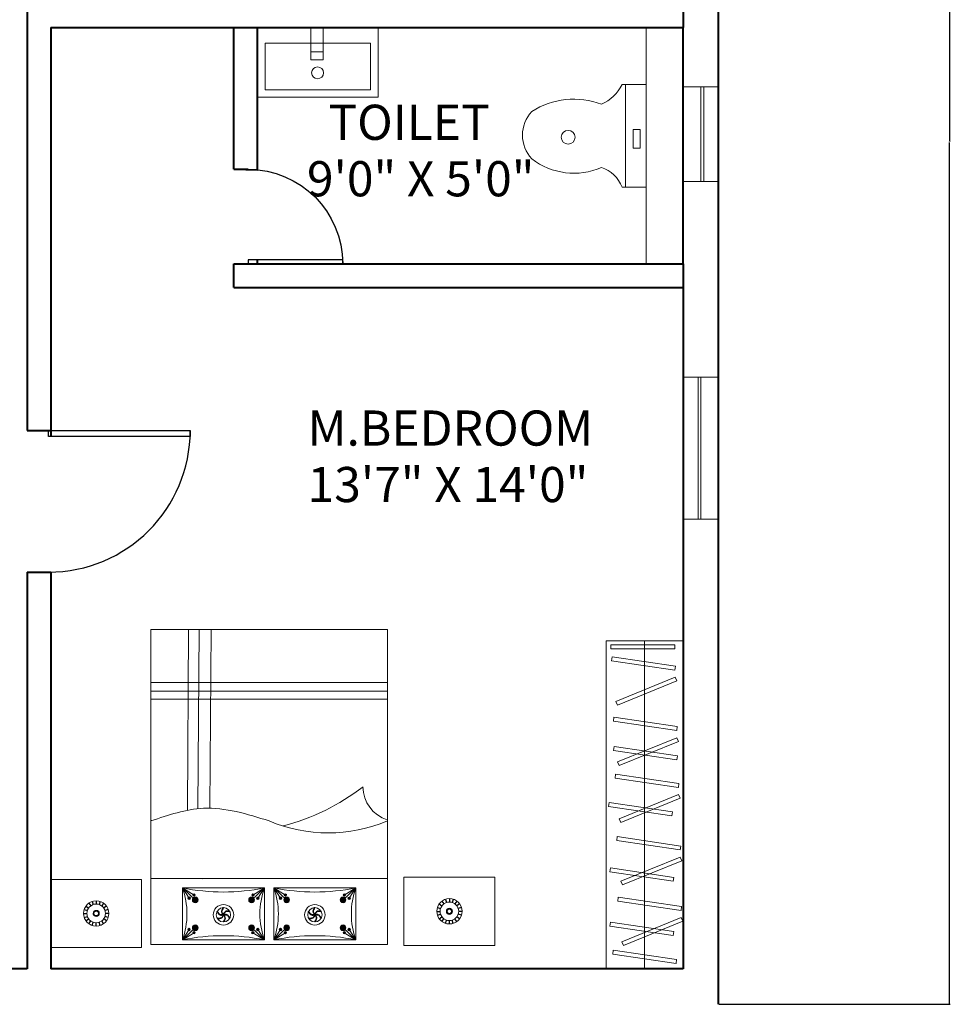
# Model space of a CAD drawing. Units: inches. Extents: x -46 to 1145, y -527 to 760.
# Tile 56 of 57: x 909 to 1145, y 222 to 472. Entities that reach past the tile are written whole.
import ezdxf

# ---------------------------------------------------------------- set-up
doc = ezdxf.new("R2010")
doc.units = ezdxf.units.IN
doc.header["$MEASUREMENT"] = 0
for name, color, linetype, lineweight in [('A-ANNO-DIMS', 2, 'Continuous', 18), ('A-AREA-IDEN', 1, 'Continuous', 18), ('A-FLOR-CASE', 32, 'Continuous', 18), ('A-FLOR-FIXT', 9, 'Continuous', 18), ('A-FURN', 2, 'Continuous', 13), ('DOORS', 3, 'Continuous', 25), ('WALLS', 4, 'Continuous', 40), ('WINDOWS', 240, 'Continuous', 20)]:
    doc.layers.add(name, color=color, linetype=linetype, lineweight=lineweight)
doc.layers.add('FURNTIURE', color=2, linetype='Continuous')
doc.layers.add('LT', color=9, linetype='Continuous')
doc.styles.get("Standard").update_dxf_attribs({"font": 'arial.ttf'})
doc.dimstyles.get("Standard").update_dxf_attribs({"dimtxt": 0.18, "dimasz": 0.18, "dimexe": 0.18, "dimexo": 0.0625, "dimgap": 0.09, "dimtad": 0, "dimtih": 1, "dimtoh": 1, "dimdec": 0, "dimzin": 0, "dimdsep": 46, "dimlunit": 3, "dimtxsty": 'Standard', "dimcen": 0.09, "dimadec": 0, "dimazin": 0, "dimtfac": 1, "dimtdec": 0, "dimtofl": 0, "dimtmove": 0, "dimatfit": 3, "dimfxl": 1, "dimtolj": 1, "dimtzin": 0, "dimarcsym": 0})

# ---------------------------------------------------------------- blocks, each defined once
blk = doc.blocks.new('*U2')
for p, q in [((0, 0), (0, -6)), ((40, 0), (40, -6))]:
    blk.add_line(p, q)
blk.add_lwpolyline([(0, 0), (0, 40), (1.75, 40), (1.75, 0)], close=True)
blk.add_arc((0, 0), 40, 0, 90)
blk = doc.blocks.new('*U89')
at = {"layer": 'FURNTIURE'}
blk.add_line((0, 0.42), (0, -0.42), dxfattribs=at)
blk = doc.blocks.new('*U90')
at = {"layer": 'FURNTIURE', "transparency": 16777216}
for p, rotation in [((590.89, 507.4), 17.99999999999997), ((592.61, 507.4), 341.9999999999999), ((589.1, 505.61), 72), ((589.5, 506.39), 54), ((590.11, 507), 36), ((593.39, 507), 324), ((594.01, 506.39), 306), ((594.4, 505.61), 288), ((588.97, 504.75), 90), ((589.1, 503.89), 108), ((589.5, 503.11), 126), ((590.11, 502.49), 144), ((590.89, 502.1), 162), ((592.61, 502.1), 197.9999999999999), ((593.39, 502.49), 216), ((594.01, 503.11), 234), ((594.4, 503.89), 252), ((594.54, 504.75), 270), ((591.75, 501.96), 180)]:
    blk.add_blockref('*U89', p, dxfattribs=dict(at, rotation=rotation))
blk.add_blockref('*U89', (591.75, 507.53), dxfattribs=at)
blk = doc.blocks.new('*U87')
at = {"layer": 'FURNTIURE'}
blk.add_line((0, 0.1), (0, -0.1), dxfattribs=at)
blk = doc.blocks.new('*U88')
at = {"layer": 'FURNTIURE', "transparency": 16777216}
for p, rotation in [((141.23, 121.04), 90), ((141.27, 121.25), 72), ((141.27, 120.83), 108), ((141.36, 121.43), 54), ((141.36, 120.65), 126), ((141.51, 121.58), 35.99999999999999), ((141.51, 120.5), 144), ((141.7, 121.67), 17.99999999999998), ((141.7, 120.4), 162), ((141.9, 120.37), 180), ((142.11, 121.67), 342), ((142.11, 120.4), 198), ((142.3, 121.58), 324), ((142.3, 120.5), 216), ((142.44, 121.43), 306), ((142.44, 120.65), 234), ((142.54, 121.25), 288), ((142.54, 120.83), 252), ((142.57, 121.04), 270)]:
    blk.add_blockref('*U87', p, dxfattribs=dict(at, rotation=rotation))
blk.add_blockref('*U87', (141.9, 121.71), dxfattribs=at)
blk = doc.blocks.new('NIGHTSTAND')
blk.add_lwpolyline([(23.06, 0), (0, 0), (0, 17.28), (23.06, 17.28)], close=True)
for radius in [3.21, 2.36, 0.77, 0.567]:
    blk.add_circle((11.53, 8.64), radius)
for name, p in [('*U90', (-580.22, -496.1)), ('*U88', (-130.37, -112.4))]:
    blk.add_blockref(name, p)
blk = doc.blocks.new('WARDROBE')
blk.add_line((9.78, 0), (9.78, 83.25))
for points in [[(19.56, 0), (0, 0), (0, 83.25), (19.56, 83.25)], [(17.74, 78.49), (1.66, 80.88), (1.8, 81.87), (17.88, 79.48)], [(15.55, 76.35), (0.49, 70.23), (0.11, 71.16), (15.17, 77.28)], [(18.43, 71.4), (2.35, 73.79), (2.5, 74.78), (18.58, 72.39)], [(16.47, 65.03), (0.39, 67.42), (0.54, 68.41), (16.62, 66.02)], [(15.79, 61), (0.73, 54.88), (0.35, 55.81), (15.41, 61.93)], [(18.43, 57.62), (2.35, 60.01), (2.5, 61), (18.58, 58.61)], [(16.71, 49.68), (0.63, 52.07), (0.78, 53.06), (16.86, 50.67)], [(16.22, 45.12), (1.16, 39), (0.78, 39.93), (15.84, 46.05)], [(18.77, 41.02), (2.69, 43.41), (2.84, 44.4), (18.92, 42.01)], [(17.14, 33.8), (1.06, 36.19), (1.21, 37.19), (17.29, 34.8)], [(16.65, 30.67), (1.59, 24.55), (1.21, 25.48), (16.27, 31.6)], [(17.52, 26.78), (1.44, 29.17), (1.59, 30.16), (17.67, 27.77)], [(17.57, 19.35), (1.49, 21.74), (1.64, 22.73), (17.72, 20.34)], [(17.08, 15.35), (2.02, 9.23), (1.64, 10.16), (16.7, 16.28)], [(18, 4.03), (1.92, 6.42), (2.07, 7.41), (18.15, 5.03)], [(18.32, 0.98), (2.07, 0.98), (2.07, 1.98), (18.32, 1.98)]]:
    blk.add_lwpolyline(points, close=True)
blk = doc.blocks.new('LAVATORY-RECT')
blk.add_line((14.01, 6.17), (17.08, 6.17))
for points in [[(30.61, 0), (0, 0), (0, 17.7), (30.61, 17.7)], [(28.7, 3.94), (1.97, 3.94), (1.97, 15.81), (28.7, 15.81)], [(17.08, 0), (14.01, 0), (14.01, 8.17), (17.08, 8.17)]]:
    blk.add_lwpolyline(points, close=True)
blk.add_circle((15.39, 11.51), 1.51)
blk = doc.blocks.new('WATER-CLOSET')
for p, q in [((0, 0), (0, 26.01)), ((0, 26.01), (6.13, 26.01)), ((5.22, 21.04), (5.22, 26.01)), ((5.22, 26.01), (5.22, 0)), ((0, 0), (6.13, 0))]:
    blk.add_line(p, q)
blk.add_lwpolyline([(1.51, 11.4), (1.51, 16.16), (3.34, 16.16), (3.34, 11.4)], close=True)
blk.add_circle((19.79, 13.37), 1.75)
for centre, radius, start, end in [((14.15, 29.2), 8.64, 201.6782, 251.0259), ((18.35, 4.96), 17.54, 52.4616, 113.5359), ((22.52, 12.84), 8.87, 317.2682, 42.7318), ((18.33, 23.71), 20, 249.5645, 302.3709), ((15.4, -4.5), 10.31, 113.1704, 154.0947)]:
    blk.add_arc(centre, radius, start, end)
blk = doc.blocks.new('WINDOW-36IN')
for p, q in [((0, 4.5), (0, 9)), ((0, 9), (0, 0)), ((36, 9), (36, 0)), ((0, 5.23), (36, 5.23)), ((0, 4.5), (36, 4.5))]:
    blk.add_line(p, q)
blk = doc.blocks.new('WINDOW-24IN')
for p, q in [((0, 4.5), (0, 9)), ((0, 9), (0, 0)), ((24, 9), (24, 0)), ((0, 5.23), (24, 5.23)), ((0, 4.5), (24, 4.5))]:
    blk.add_line(p, q)
blk = doc.blocks.new('*U58')
at = {"layer": 'LT'}
blk.add_line((0, 0.28), (0, -0.28), dxfattribs=at)
for centre, start, end in [((0.73, 0), 159.0676, 200.9324), ((-0.73, 0), 339.0676, 20.9324)]:
    blk.add_arc(centre, 0.786, start, end, dxfattribs=at)
blk = doc.blocks.new('*U59')
at = {"layer": 'LT', "transparency": 16777216}
for p, rotation in [((609.66, 443.79), 80.00000000000001), ((609.69, 443.6), 120), ((609.76, 443.96), 40.00000000000002), ((609.84, 443.48), 160), ((610.03, 443.48), 200), ((610.12, 443.96), 320), ((610.18, 443.6), 240), ((610.21, 443.79), 280)]:
    blk.add_blockref('*U58', p, dxfattribs=dict(at, rotation=rotation))
blk.add_blockref('*U58', (609.94, 444.03), dxfattribs=at)
blk = doc.blocks.new('*U60')
at = {"layer": 'LT'}
blk.add_line((0, 0.12), (0, -0.12), dxfattribs=at)
for centre, start, end in [((0.31, 0), 159.0676, 200.9324), ((-0.31, 0), 339.0676, 20.9324)]:
    blk.add_arc(centre, 0.335, start, end, dxfattribs=at)
blk = doc.blocks.new('*U61')
at = {"layer": 'LT', "transparency": 16777216}
for p, rotation in [((259.5, 188.9), 80.00000000000001), ((259.51, 188.82), 120), ((259.54, 188.97), 40), ((259.57, 188.76), 160), ((259.65, 188.76), 200), ((259.69, 188.97), 320), ((259.72, 188.82), 240), ((259.73, 188.9), 280)]:
    blk.add_blockref('*U60', p, dxfattribs=dict(at, rotation=rotation))
blk.add_blockref('*U60', (259.61, 189), dxfattribs=at)
blk = doc.blocks.new('*U62')
at = {"layer": 'LT'}
blk.add_line((0, 0.12), (0, -0.12), dxfattribs=at)
for centre, start, end in [((0.31, 0), 159.0676, 200.9324), ((-0.31, 0), 339.0676, 20.9324)]:
    blk.add_arc(centre, 0.335, start, end, dxfattribs=at)
blk = doc.blocks.new('*U63')
at = {"layer": 'LT', "transparency": 16777216}
for p, rotation in [((259.5, 188.9), 80.00000000000001), ((259.51, 188.82), 120), ((259.54, 188.97), 40), ((259.57, 188.76), 160), ((259.65, 188.76), 200), ((259.69, 188.97), 320), ((259.72, 188.82), 240), ((259.73, 188.9), 280)]:
    blk.add_blockref('*U62', p, dxfattribs=dict(at, rotation=rotation))
blk.add_blockref('*U62', (259.61, 189), dxfattribs=at)
blk = doc.blocks.new('*U64')
at = {"layer": 'LT'}
blk.add_line((0, 0.28), (0, -0.28), dxfattribs=at)
for centre, start, end in [((0.73, 0), 159.0676, 200.9324), ((-0.73, 0), 339.0676, 20.9324)]:
    blk.add_arc(centre, 0.786, start, end, dxfattribs=at)
blk = doc.blocks.new('*U65')
at = {"layer": 'LT', "transparency": 16777216}
for p, rotation in [((609.66, 443.79), 80.00000000000001), ((609.69, 443.6), 120), ((609.76, 443.96), 40.00000000000002), ((609.84, 443.48), 160), ((610.03, 443.48), 200), ((610.12, 443.96), 320), ((610.18, 443.6), 240), ((610.21, 443.79), 280)]:
    blk.add_blockref('*U64', p, dxfattribs=dict(at, rotation=rotation))
blk.add_blockref('*U64', (609.94, 444.03), dxfattribs=at)
blk = doc.blocks.new('*U66')
at = {"layer": 'LT'}
blk.add_line((0, 0.12), (0, -0.12), dxfattribs=at)
for centre, start, end in [((0.31, 0), 159.0676, 200.9324), ((-0.31, 0), 339.0676, 20.9324)]:
    blk.add_arc(centre, 0.335, start, end, dxfattribs=at)
blk = doc.blocks.new('*U67')
at = {"layer": 'LT', "transparency": 16777216}
for p, rotation in [((259.5, 188.9), 80.00000000000001), ((259.51, 188.82), 120), ((259.54, 188.97), 40), ((259.57, 188.76), 160), ((259.65, 188.76), 200), ((259.69, 188.97), 320), ((259.72, 188.82), 240), ((259.73, 188.9), 280)]:
    blk.add_blockref('*U66', p, dxfattribs=dict(at, rotation=rotation))
blk.add_blockref('*U66', (259.61, 189), dxfattribs=at)
blk = doc.blocks.new('*U68')
at = {"layer": 'LT'}
blk.add_line((0, 0.12), (0, -0.12), dxfattribs=at)
for centre, start, end in [((0.31, 0), 159.0676, 200.9324), ((-0.31, 0), 339.0676, 20.9324)]:
    blk.add_arc(centre, 0.335, start, end, dxfattribs=at)
blk = doc.blocks.new('*U69')
at = {"layer": 'LT', "transparency": 16777216}
for p, rotation in [((259.5, 188.9), 80.00000000000001), ((259.51, 188.82), 120), ((259.54, 188.97), 40), ((259.57, 188.76), 160), ((259.65, 188.76), 200), ((259.69, 188.97), 320), ((259.72, 188.82), 240), ((259.73, 188.9), 280)]:
    blk.add_blockref('*U68', p, dxfattribs=dict(at, rotation=rotation))
blk.add_blockref('*U68', (259.61, 189), dxfattribs=at)
blk = doc.blocks.new('*U70')
at = {"layer": 'LT'}
blk.add_line((0, 0.28), (0, -0.28), dxfattribs=at)
for centre, start, end in [((0.73, 0), 159.0676, 200.9324), ((-0.73, 0), 339.0676, 20.9324)]:
    blk.add_arc(centre, 0.786, start, end, dxfattribs=at)
blk = doc.blocks.new('*U71')
at = {"layer": 'LT', "transparency": 16777216}
for p, rotation in [((609.66, 443.79), 80.00000000000001), ((609.69, 443.6), 120), ((609.76, 443.96), 40.00000000000002), ((609.84, 443.48), 160), ((610.03, 443.48), 200), ((610.12, 443.96), 320), ((610.18, 443.6), 240), ((610.21, 443.79), 280)]:
    blk.add_blockref('*U70', p, dxfattribs=dict(at, rotation=rotation))
blk.add_blockref('*U70', (609.94, 444.03), dxfattribs=at)
blk = doc.blocks.new('*U46')
at = {"layer": 'LT'}
blk.add_line((0, 0.12), (0, -0.12), dxfattribs=at)
for centre, start, end in [((0.31, 0), 159.0676, 200.9324), ((-0.31, 0), 339.0676, 20.9324)]:
    blk.add_arc(centre, 0.335, start, end, dxfattribs=at)
blk = doc.blocks.new('*U47')
at = {"layer": 'LT', "transparency": 16777216}
for p, rotation in [((259.5, 188.9), 80.00000000000001), ((259.51, 188.82), 120), ((259.54, 188.97), 40), ((259.57, 188.76), 160), ((259.65, 188.76), 200), ((259.69, 188.97), 320), ((259.72, 188.82), 240), ((259.73, 188.9), 280)]:
    blk.add_blockref('*U46', p, dxfattribs=dict(at, rotation=rotation))
blk.add_blockref('*U46', (259.61, 189), dxfattribs=at)
blk = doc.blocks.new('*U48')
at = {"layer": 'LT'}
blk.add_line((0, 0.12), (0, -0.12), dxfattribs=at)
for centre, start, end in [((0.31, 0), 159.0676, 200.9324), ((-0.31, 0), 339.0676, 20.9324)]:
    blk.add_arc(centre, 0.335, start, end, dxfattribs=at)
blk = doc.blocks.new('*U49')
at = {"layer": 'LT', "transparency": 16777216}
for p, rotation in [((259.5, 188.9), 80.00000000000001), ((259.51, 188.82), 120), ((259.54, 188.97), 40), ((259.57, 188.76), 160), ((259.65, 188.76), 200), ((259.69, 188.97), 320), ((259.72, 188.82), 240), ((259.73, 188.9), 280)]:
    blk.add_blockref('*U48', p, dxfattribs=dict(at, rotation=rotation))
blk.add_blockref('*U48', (259.61, 189), dxfattribs=at)
blk = doc.blocks.new('*U50')
at = {"layer": 'LT'}
blk.add_line((0, 0.28), (0, -0.28), dxfattribs=at)
for centre, start, end in [((0.73, 0), 159.0676, 200.9324), ((-0.73, 0), 339.0676, 20.9324)]:
    blk.add_arc(centre, 0.786, start, end, dxfattribs=at)
blk = doc.blocks.new('*U51')
at = {"layer": 'LT', "transparency": 16777216}
for p, rotation in [((609.66, 443.79), 80.00000000000001), ((609.69, 443.6), 120), ((609.76, 443.96), 40.00000000000002), ((609.84, 443.48), 160), ((610.03, 443.48), 200), ((610.12, 443.96), 320), ((610.18, 443.6), 240), ((610.21, 443.79), 280)]:
    blk.add_blockref('*U50', p, dxfattribs=dict(at, rotation=rotation))
blk.add_blockref('*U50', (609.94, 444.03), dxfattribs=at)
blk = doc.blocks.new('*U52')
at = {"layer": 'LT'}
blk.add_line((0, 0.12), (0, -0.12), dxfattribs=at)
for centre, start, end in [((0.31, 0), 159.0676, 200.9324), ((-0.31, 0), 339.0676, 20.9324)]:
    blk.add_arc(centre, 0.335, start, end, dxfattribs=at)
blk = doc.blocks.new('*U53')
at = {"layer": 'LT', "transparency": 16777216}
for p, rotation in [((259.5, 188.9), 80.00000000000001), ((259.51, 188.82), 120), ((259.54, 188.97), 40), ((259.57, 188.76), 160), ((259.65, 188.76), 200), ((259.69, 188.97), 320), ((259.72, 188.82), 240), ((259.73, 188.9), 280)]:
    blk.add_blockref('*U52', p, dxfattribs=dict(at, rotation=rotation))
blk.add_blockref('*U52', (259.61, 189), dxfattribs=at)
blk = doc.blocks.new('*U54')
at = {"layer": 'LT'}
blk.add_line((0, 0.12), (0, -0.12), dxfattribs=at)
for centre, start, end in [((0.31, 0), 159.0676, 200.9324), ((-0.31, 0), 339.0676, 20.9324)]:
    blk.add_arc(centre, 0.335, start, end, dxfattribs=at)
blk = doc.blocks.new('*U55')
at = {"layer": 'LT', "transparency": 16777216}
for p, rotation in [((259.5, 188.9), 80.00000000000001), ((259.51, 188.82), 120), ((259.54, 188.97), 40), ((259.57, 188.76), 160), ((259.65, 188.76), 200), ((259.69, 188.97), 320), ((259.72, 188.82), 240), ((259.73, 188.9), 280)]:
    blk.add_blockref('*U54', p, dxfattribs=dict(at, rotation=rotation))
blk.add_blockref('*U54', (259.61, 189), dxfattribs=at)
blk = doc.blocks.new('*U34')
at = {"layer": 'LT'}
blk.add_line((0, 0.28), (0, -0.28), dxfattribs=at)
for centre, start, end in [((0.73, 0), 159.0676, 200.9324), ((-0.73, 0), 339.0676, 20.9324)]:
    blk.add_arc(centre, 0.786, start, end, dxfattribs=at)
blk = doc.blocks.new('*U35')
at = {"layer": 'LT', "transparency": 16777216}
for p, rotation in [((609.66, 443.79), 80.00000000000001), ((609.69, 443.6), 120), ((609.76, 443.96), 40.00000000000002), ((609.84, 443.48), 160), ((610.03, 443.48), 200), ((610.12, 443.96), 320), ((610.18, 443.6), 240), ((610.21, 443.79), 280)]:
    blk.add_blockref('*U34', p, dxfattribs=dict(at, rotation=rotation))
blk.add_blockref('*U34', (609.94, 444.03), dxfattribs=at)
blk = doc.blocks.new('*U36')
at = {"layer": 'LT'}
blk.add_line((0, 0.12), (0, -0.12), dxfattribs=at)
for centre, start, end in [((0.31, 0), 159.0676, 200.9324), ((-0.31, 0), 339.0676, 20.9324)]:
    blk.add_arc(centre, 0.335, start, end, dxfattribs=at)
blk = doc.blocks.new('*U37')
at = {"layer": 'LT', "transparency": 16777216}
for p, rotation in [((259.5, 188.9), 80.00000000000001), ((259.51, 188.82), 120), ((259.54, 188.97), 40), ((259.57, 188.76), 160), ((259.65, 188.76), 200), ((259.69, 188.97), 320), ((259.72, 188.82), 240), ((259.73, 188.9), 280)]:
    blk.add_blockref('*U36', p, dxfattribs=dict(at, rotation=rotation))
blk.add_blockref('*U36', (259.61, 189), dxfattribs=at)
blk = doc.blocks.new('*U38')
at = {"layer": 'LT'}
blk.add_line((0, 0.12), (0, -0.12), dxfattribs=at)
for centre, start, end in [((0.31, 0), 159.0676, 200.9324), ((-0.31, 0), 339.0676, 20.9324)]:
    blk.add_arc(centre, 0.335, start, end, dxfattribs=at)
blk = doc.blocks.new('*U39')
at = {"layer": 'LT', "transparency": 16777216}
for p, rotation in [((259.5, 188.9), 80.00000000000001), ((259.51, 188.82), 120), ((259.54, 188.97), 40), ((259.57, 188.76), 160), ((259.65, 188.76), 200), ((259.69, 188.97), 320), ((259.72, 188.82), 240), ((259.73, 188.9), 280)]:
    blk.add_blockref('*U38', p, dxfattribs=dict(at, rotation=rotation))
blk.add_blockref('*U38', (259.61, 189), dxfattribs=at)
blk = doc.blocks.new('*U40')
at = {"layer": 'LT'}
blk.add_line((0, 0.28), (0, -0.28), dxfattribs=at)
for centre, start, end in [((0.73, 0), 159.0676, 200.9324), ((-0.73, 0), 339.0676, 20.9324)]:
    blk.add_arc(centre, 0.786, start, end, dxfattribs=at)
blk = doc.blocks.new('*U41')
at = {"layer": 'LT', "transparency": 16777216}
for p, rotation in [((609.66, 443.79), 80.00000000000001), ((609.69, 443.6), 120), ((609.76, 443.96), 40.00000000000002), ((609.84, 443.48), 160), ((610.03, 443.48), 200), ((610.12, 443.96), 320), ((610.18, 443.6), 240), ((610.21, 443.79), 280)]:
    blk.add_blockref('*U40', p, dxfattribs=dict(at, rotation=rotation))
blk.add_blockref('*U40', (609.94, 444.03), dxfattribs=at)
blk = doc.blocks.new('*U42')
at = {"layer": 'LT'}
blk.add_line((0, 0.12), (0, -0.12), dxfattribs=at)
for centre, start, end in [((0.31, 0), 159.0676, 200.9324), ((-0.31, 0), 339.0676, 20.9324)]:
    blk.add_arc(centre, 0.335, start, end, dxfattribs=at)
blk = doc.blocks.new('*U43')
at = {"layer": 'LT', "transparency": 16777216}
for p, rotation in [((259.5, 188.9), 80.00000000000001), ((259.51, 188.82), 120), ((259.54, 188.97), 40), ((259.57, 188.76), 160), ((259.65, 188.76), 200), ((259.69, 188.97), 320), ((259.72, 188.82), 240), ((259.73, 188.9), 280)]:
    blk.add_blockref('*U42', p, dxfattribs=dict(at, rotation=rotation))
blk.add_blockref('*U42', (259.61, 189), dxfattribs=at)
blk = doc.blocks.new('*U44')
at = {"layer": 'LT'}
blk.add_line((0, 0.12), (0, -0.12), dxfattribs=at)
for centre, start, end in [((0.31, 0), 159.0676, 200.9324), ((-0.31, 0), 339.0676, 20.9324)]:
    blk.add_arc(centre, 0.335, start, end, dxfattribs=at)
blk = doc.blocks.new('*U45')
at = {"layer": 'LT', "transparency": 16777216}
for p, rotation in [((259.5, 188.9), 80.00000000000001), ((259.51, 188.82), 120), ((259.54, 188.97), 40), ((259.57, 188.76), 160), ((259.65, 188.76), 200), ((259.69, 188.97), 320), ((259.72, 188.82), 240), ((259.73, 188.9), 280)]:
    blk.add_blockref('*U44', p, dxfattribs=dict(at, rotation=rotation))
blk.add_blockref('*U44', (259.61, 189), dxfattribs=at)
blk = doc.blocks.new('*U72')
at = {"layer": 'LT'}
blk.add_line((0, 0.28), (0, -0.28), dxfattribs=at)
for centre, start, end in [((0.73, 0), 159.0676, 200.9324), ((-0.73, 0), 339.0676, 20.9324)]:
    blk.add_arc(centre, 0.786, start, end, dxfattribs=at)
blk = doc.blocks.new('*U73')
at = {"layer": 'LT', "transparency": 16777216}
for p, rotation in [((609.66, 443.79), 80.00000000000001), ((609.69, 443.6), 120), ((609.76, 443.96), 40.00000000000002), ((609.84, 443.48), 160), ((610.03, 443.48), 200), ((610.12, 443.96), 320), ((610.18, 443.6), 240), ((610.21, 443.79), 280)]:
    blk.add_blockref('*U72', p, dxfattribs=dict(at, rotation=rotation))
blk.add_blockref('*U72', (609.94, 444.03), dxfattribs=at)
blk = doc.blocks.new('*U74')
at = {"layer": 'LT'}
blk.add_line((0, 0.12), (0, -0.12), dxfattribs=at)
for centre, start, end in [((0.31, 0), 159.0676, 200.9324), ((-0.31, 0), 339.0676, 20.9324)]:
    blk.add_arc(centre, 0.335, start, end, dxfattribs=at)
blk = doc.blocks.new('*U75')
at = {"layer": 'LT', "transparency": 16777216}
for p, rotation in [((259.5, 188.9), 80.00000000000001), ((259.51, 188.82), 120), ((259.54, 188.97), 40), ((259.57, 188.76), 160), ((259.65, 188.76), 200), ((259.69, 188.97), 320), ((259.72, 188.82), 240), ((259.73, 188.9), 280)]:
    blk.add_blockref('*U74', p, dxfattribs=dict(at, rotation=rotation))
blk.add_blockref('*U74', (259.61, 189), dxfattribs=at)
blk = doc.blocks.new('*U76')
at = {"layer": 'LT'}
blk.add_line((0, 0.12), (0, -0.12), dxfattribs=at)
for centre, start, end in [((0.31, 0), 159.0676, 200.9324), ((-0.31, 0), 339.0676, 20.9324)]:
    blk.add_arc(centre, 0.335, start, end, dxfattribs=at)
blk = doc.blocks.new('*U77')
at = {"layer": 'LT', "transparency": 16777216}
for p, rotation in [((259.5, 188.9), 80.00000000000001), ((259.51, 188.82), 120), ((259.54, 188.97), 40), ((259.57, 188.76), 160), ((259.65, 188.76), 200), ((259.69, 188.97), 320), ((259.72, 188.82), 240), ((259.73, 188.9), 280)]:
    blk.add_blockref('*U76', p, dxfattribs=dict(at, rotation=rotation))
blk.add_blockref('*U76', (259.61, 189), dxfattribs=at)
blk = doc.blocks.new('*U78')
at = {"layer": 'LT'}
blk.add_line((0, 0.28), (0, -0.28), dxfattribs=at)
for centre, start, end in [((0.73, 0), 159.0676, 200.9324), ((-0.73, 0), 339.0676, 20.9324)]:
    blk.add_arc(centre, 0.786, start, end, dxfattribs=at)
blk = doc.blocks.new('*U79')
at = {"layer": 'LT', "transparency": 16777216}
for p, rotation in [((609.66, 443.79), 80.00000000000001), ((609.69, 443.6), 120), ((609.76, 443.96), 40.00000000000002), ((609.84, 443.48), 160), ((610.03, 443.48), 200), ((610.12, 443.96), 320), ((610.18, 443.6), 240), ((610.21, 443.79), 280)]:
    blk.add_blockref('*U78', p, dxfattribs=dict(at, rotation=rotation))
blk.add_blockref('*U78', (609.94, 444.03), dxfattribs=at)
blk = doc.blocks.new('*U80')
at = {"layer": 'LT'}
blk.add_line((0, 0.12), (0, -0.12), dxfattribs=at)
for centre, start, end in [((0.31, 0), 159.0676, 200.9324), ((-0.31, 0), 339.0676, 20.9324)]:
    blk.add_arc(centre, 0.335, start, end, dxfattribs=at)
blk = doc.blocks.new('*U81')
at = {"layer": 'LT', "transparency": 16777216}
for p, rotation in [((259.5, 188.9), 80.00000000000001), ((259.51, 188.82), 120), ((259.54, 188.97), 40), ((259.57, 188.76), 160), ((259.65, 188.76), 200), ((259.69, 188.97), 320), ((259.72, 188.82), 240), ((259.73, 188.9), 280)]:
    blk.add_blockref('*U80', p, dxfattribs=dict(at, rotation=rotation))
blk.add_blockref('*U80', (259.61, 189), dxfattribs=at)
blk = doc.blocks.new('*U82')
at = {"layer": 'LT'}
blk.add_line((0, 0.12), (0, -0.12), dxfattribs=at)
for centre, start, end in [((0.31, 0), 159.0676, 200.9324), ((-0.31, 0), 339.0676, 20.9324)]:
    blk.add_arc(centre, 0.335, start, end, dxfattribs=at)
blk = doc.blocks.new('*U83')
at = {"layer": 'LT', "transparency": 16777216}
for p, rotation in [((259.5, 188.9), 80.00000000000001), ((259.51, 188.82), 120), ((259.54, 188.97), 40), ((259.57, 188.76), 160), ((259.65, 188.76), 200), ((259.69, 188.97), 320), ((259.72, 188.82), 240), ((259.73, 188.9), 280)]:
    blk.add_blockref('*U82', p, dxfattribs=dict(at, rotation=rotation))
blk.add_blockref('*U82', (259.61, 189), dxfattribs=at)
blk = doc.blocks.new('*U32')
at = {"layer": 'FURNTIURE'}
blk.add_open_spline([(0.04, 1.82), (-0.22, 1.45), (-0.66, 0.8), (0.1, -0.02), (0.64, -0.93), (0.24, -1.53), (0.04, -1.82)], degree=3, knots=[0, 0, 0, 0, 1.177175, 2.037162, 3.056205, 4.032246, 4.032246, 4.032246, 4.032246], dxfattribs=at)
blk = doc.blocks.new('*U33')
at = {"layer": 'FURNTIURE', "transparency": 16777216}
blk.add_blockref('*U32', (904.3, 663.38), dxfattribs=at)
for p, rotation in [((904.38, 663.38), 180), ((904.32, 663.42), 300), ((904.32, 663.35), 59.99999999999999), ((904.36, 663.42), 239.9999999999999), ((904.36, 663.35), 119.9999999999999)]:
    blk.add_blockref('*U32', p, dxfattribs=dict(at, rotation=rotation))
blk = doc.blocks.new('*U56')
at = {"layer": 'FURNTIURE'}
blk.add_open_spline([(0.04, 1.82), (-0.22, 1.45), (-0.66, 0.8), (0.1, -0.02), (0.64, -0.93), (0.24, -1.53), (0.04, -1.82)], degree=3, knots=[0, 0, 0, 0, 1.177175, 2.037162, 3.056205, 4.032246, 4.032246, 4.032246, 4.032246], dxfattribs=at)
blk = doc.blocks.new('*U57')
at = {"layer": 'FURNTIURE', "transparency": 16777216}
blk.add_blockref('*U56', (904.3, 663.38), dxfattribs=at)
for p, rotation in [((904.38, 663.38), 180), ((904.32, 663.42), 300), ((904.32, 663.35), 59.99999999999999), ((904.36, 663.42), 239.9999999999999), ((904.36, 663.35), 119.9999999999999)]:
    blk.add_blockref('*U56', p, dxfattribs=dict(at, rotation=rotation))
blk = doc.blocks.new('BED-QUEEN-FURNISHED')
for p, q in [((0, 0), (0, 80)), ((0, 80), (60, 80)), ((60, 80), (60, 0)), ((8, 78.8), (28.8, 78.8)), ((8, 65.6), (8, 78.8)), ((8, 78.8), (11.38, 75.61)), ((8, 78.8), (9.68, 76.18)), ((8, 78.8), (10.93, 76.98)), ((28.8, 78.8), (25.41, 75.61)), ((28.8, 78.8), (25.87, 76.98)), ((28.8, 78.8), (27.12, 76.18)), ((28.8, 78.8), (28.8, 65.6)), ((31.2, 78.8), (52, 78.8)), ((31.2, 65.6), (31.2, 78.8)), ((31.2, 78.8), (52, 78.8)), ((31.2, 65.6), (31.2, 78.8)), ((31.2, 78.8), (34.58, 75.61)), ((31.2, 78.8), (32.88, 76.18)), ((31.2, 78.8), (34.13, 76.98)), ((52, 78.8), (48.61, 75.61)), ((52, 78.8), (49.07, 76.98)), ((52, 78.8), (50.32, 76.18)), ((52, 78.8), (52, 65.6)), ((52, 78.8), (52, 65.6)), ((10.93, 76.98), (10.93, 76.75)), ((11.25, 75.74), (11.25, 75.18)), ((25.55, 75.74), (25.55, 75.18)), ((25.87, 76.98), (25.87, 76.75)), ((27.12, 76.18), (27.12, 75.95)), ((34.13, 76.98), (34.13, 76.75)), ((34.45, 75.74), (34.45, 75.18)), ((48.75, 75.74), (48.75, 75.18)), ((49.07, 76.98), (49.07, 76.75)), ((50.32, 76.18), (50.32, 75.95)), ((8, 65.61), (11.38, 68.8)), ((8, 65.61), (9.68, 68.23)), ((10.92, 67.43), (10.92, 67.67)), ((11.25, 68.67), (11.25, 69.23)), ((28.8, 65.6), (25.41, 68.79)), ((25.87, 67.42), (25.87, 67.66)), ((27.11, 68.22), (27.11, 68.46)), ((28.8, 65.6), (27.11, 68.22)), ((31.2, 65.61), (34.58, 68.8)), ((31.2, 65.61), (32.88, 68.23)), ((34.12, 67.43), (34.12, 67.67)), ((34.45, 68.67), (34.45, 69.23)), ((52, 65.6), (48.61, 68.79)), ((49.07, 67.42), (49.07, 67.66)), ((50.31, 68.22), (50.31, 68.46)), ((52, 65.6), (50.31, 68.22)), ((8, 65.61), (10.92, 67.43)), ((8, 65.6), (28.8, 65.6)), ((28.8, 65.6), (25.87, 67.42)), ((31.2, 65.61), (34.12, 67.43)), ((31.2, 65.6), (52, 65.6)), ((31.2, 65.6), (52, 65.6)), ((52, 65.6), (49.07, 67.42)), ((60, 63.2), (0, 63.2)), ((46.8, 63.6), (46.8, 63.6)), ((44.72, 0), (45.02, 45.37)), ((47.8, 0), (48.1, 45.5)), ((50.46, 0), (50.76, 45.91)), ((0, 17.7), (60, 17.7)), ((0, 15.69), (60, 15.69)), ((0, 13.42), (60, 13.42)), ((60, 0), (0, 0))]:
    blk.add_line(p, q)
for centre, radius in [((9.68, 76.18), 0.308), ((9.68, 76.18), 0.239), ((11.25, 75.74), 0.723), ((10.93, 76.98), 0.308), ((10.93, 76.98), 0.239), ((11.25, 75.74), 0.562), ((18.4, 72.44), 2.6), ((25.55, 75.74), 0.723), ((25.55, 75.74), 0.562), ((25.87, 76.98), 0.308), ((25.87, 76.98), 0.239), ((27.12, 76.18), 0.308), ((27.12, 76.18), 0.239), ((32.88, 76.18), 0.308), ((32.88, 76.18), 0.239), ((34.45, 75.74), 0.723), ((34.13, 76.98), 0.308), ((34.13, 76.98), 0.239), ((34.45, 75.74), 0.562), ((41.6, 72.44), 2.6), ((48.75, 75.74), 0.723), ((48.75, 75.74), 0.562), ((49.07, 76.98), 0.308), ((49.07, 76.98), 0.239), ((50.32, 76.18), 0.308), ((50.32, 76.18), 0.239), ((18.4, 72.44), 1.82), ((41.6, 72.44), 1.82), ((9.68, 68.23), 0.308), ((9.68, 68.23), 0.239), ((11.25, 68.67), 0.723), ((10.92, 67.43), 0.308), ((10.92, 67.43), 0.239), ((11.25, 68.67), 0.562), ((25.55, 68.66), 0.723), ((25.55, 68.66), 0.562), ((25.87, 67.42), 0.308), ((25.87, 67.42), 0.239), ((27.11, 68.22), 0.308), ((27.11, 68.22), 0.239), ((32.88, 68.23), 0.308), ((32.88, 68.23), 0.239), ((34.45, 68.67), 0.723), ((34.12, 67.43), 0.308), ((34.12, 67.43), 0.239), ((34.45, 68.67), 0.562), ((48.75, 68.66), 0.723), ((48.75, 68.66), 0.562), ((49.07, 67.42), 0.308), ((49.07, 67.42), 0.239), ((50.31, 68.22), 0.308), ((50.31, 68.22), 0.239)]:
    blk.add_circle(centre, radius)
for centre, radius, start, end in [((18.4, 129.18), 51.44, 258.3356, 281.6644), ((-10.65, 72.2), 19.79, 340.5151, 19.4849), ((47.45, 72.2), 19.79, 160.5151, 199.4849), ((41.6, 129.18), 51.44, 258.3356, 281.6644), ((12.55, 72.2), 19.79, 340.5151, 19.4849), ((70.65, 72.2), 19.79, 160.5151, 199.4849), ((11.24, 76.86), 0.335, 159.0676, 200.9324), ((10.61, 76.86), 0.335, 339.0676, 20.9324), ((11.99, 75.46), 0.786, 159.0676, 200.9324), ((10.52, 75.46), 0.786, 339.0676, 20.9324), ((26.28, 75.46), 0.786, 159.0676, 200.9324), ((24.81, 75.46), 0.786, 339.0676, 20.9324), ((26.19, 76.86), 0.335, 159.0676, 200.9324), ((25.56, 76.86), 0.335, 339.0676, 20.9324), ((27.43, 76.06), 0.335, 159.0676, 200.9324), ((26.8, 76.06), 0.335, 339.0676, 20.9324), ((34.44, 76.86), 0.335, 159.0676, 200.9324), ((33.81, 76.86), 0.335, 339.0676, 20.9324), ((35.19, 75.46), 0.786, 159.0676, 200.9324), ((33.72, 75.46), 0.786, 339.0676, 20.9324), ((49.48, 75.46), 0.786, 159.0676, 200.9324), ((48.01, 75.46), 0.786, 339.0676, 20.9324), ((49.39, 76.86), 0.335, 159.0676, 200.9324), ((48.76, 76.86), 0.335, 339.0676, 20.9324), ((50.63, 76.06), 0.335, 159.0676, 200.9324), ((50, 76.06), 0.335, 339.0676, 20.9324), ((11.24, 67.55), 0.335, 159.028, 200.8928), ((10.61, 67.55), 0.335, 339.028, 20.8928), ((11.98, 68.95), 0.786, 159.028, 200.8928), ((10.51, 68.95), 0.786, 339.028, 20.8928), ((26.18, 67.54), 0.335, 159.028, 200.8928), ((25.56, 67.54), 0.335, 339.028, 20.8928), ((27.43, 68.34), 0.335, 159.028, 200.8928), ((26.8, 68.34), 0.335, 339.028, 20.8928), ((34.44, 67.55), 0.335, 159.028, 200.8928), ((33.81, 67.55), 0.335, 339.028, 20.8928), ((35.18, 68.95), 0.786, 159.028, 200.8928), ((33.71, 68.95), 0.786, 339.028, 20.8928), ((49.38, 67.54), 0.335, 159.028, 200.8928), ((48.76, 67.54), 0.335, 339.028, 20.8928), ((50.63, 68.34), 0.335, 159.028, 200.8928), ((50, 68.34), 0.335, 339.028, 20.8928), ((18.4, 15.22), 51.44, 78.3356, 101.6644), ((41.6, 15.22), 51.44, 78.3356, 101.6644), ((15, 13.08), 38.56, 67.1089, 112.8911), ((-2.62, 39.94), 8.8, 0, 72.6522), ((40.88, -5.13), 56.88, 104.6834, 127.6009), ((40.88, -5.13), 56.88, 70.3635, 70.606)]:
    blk.add_arc(centre, radius, start, end)
blk.add_open_spline([(30, 48.6), (35.57, 46.87), (45.64, 43.74), (55.56, 47.1), (60, 48.6)], degree=3, knots=[0, 0, 0, 0, 16.971495, 30.687365, 30.687365, 30.687365, 30.687365])
at = {"xscale": -1}
for name, p in [('*U43', (269.3, -112.69)), ('*U45', (270.54, -111.89)), ('*U41', (621.19, -368.01)), ('*U67', (292.5, -112.69)), ('*U69', (293.74, -111.89)), ('*U65', (644.39, -368.01))]:
    blk.add_blockref(name, p, dxfattribs=at)
for name, p in [('*U35', (-584.39, -368.01)), ('*U39', (-233.74, -111.89)), ('*U37', (-232.5, -112.69)), ('*U59', (-561.19, -368.01)), ('*U63', (-210.54, -111.89)), ('*U61', (-209.3, -112.69)), ('*U33', (-885.94, -590.95)), ('*U57', (-862.74, -590.95))]:
    blk.add_blockref(name, p)
at = {"rotation": 179.9603994254766}
for name, p in [('*U81', (269.43, 256.92)), ('*U83', (270.67, 256.12)), ('*U79', (621.49, 512)), ('*U53', (292.63, 256.92)), ('*U55', (293.87, 256.12)), ('*U51', (644.69, 512))]:
    blk.add_blockref(name, p, dxfattribs=at)
at = {"xscale": -1, "rotation": 179.9603994254766}
for name, p in [('*U73', (-584.08, 512.83)), ('*U77', (-233.61, 256.47)), ('*U75', (-232.37, 257.27)), ('*U71', (-560.88, 512.83)), ('*U49', (-210.41, 256.47)), ('*U47', (-209.17, 257.27))]:
    blk.add_blockref(name, p, dxfattribs=at)
blk = doc.blocks.new('*D688')
at = {"layer": 'A-ANNO-DIMS', "color": 0, "lineweight": -2, "transparency": 16777216}
for p, q in [((1086.63, 659.52), (1145.34, 659.52)), ((1145.16, 659.34), (1145.16, 440.7)), ((1145.16, 221.7), (1145.16, 440.34)), ((1086.63, 221.52), (1145.34, 221.52))]:
    blk.add_line(p, q, dxfattribs=at)
at = {"layer": 'A-ANNO-DIMS', "color": 0, "transparency": 16777216}
for points in [[(1145.13, 659.34), (1145.19, 659.34), (1145.16, 659.52)], [(1145.13, 221.7), (1145.19, 221.7), (1145.16, 221.52)]]:
    blk.add_solid(points, dxfattribs=at)
at = {"layer": 'Defpoints', "color": 0, "transparency": 16777216}
for p in [(1086.56, 659.52), (1145.16, 659.52), (1086.56, 221.52)]:
    blk.add_point(p, dxfattribs=at)
at = {"layer": 'A-ANNO-DIMS', "color": 0, "transparency": 16777216, "insert": (1145.16, 440.52), "char_height": 0.18, "attachment_point": 5}
blk.add_mtext('\\A1;438', dxfattribs=at)

msp = doc.modelspace()

# ---------------------------------------------------------------- linework, layer by layer
at = {"layer": 'A-FLOR-CASE'}
msp.add_line((1068.1812, 409.5176), (1068.1812, 469.5176), dxfattribs=at)
at = {"layer": 'WALLS'}
for p, q in [((1086.5637, 221.5176), (1086.5637, 659.5176)), ((911.0637, 475.5176), (911.0637, 367.232)), ((1077.5637, 475.5176), (1077.5637, 469.5176)), ((917.0637, 469.5176), (917.0637, 365.657)), ((917.0637, 469.5176), (1077.5637, 469.5176)), ((963.5637, 433.5176), (963.5637, 469.5176)), ((969.5637, 433.3973), (969.5637, 469.5176)), ((1077.5637, 409.5176), (1077.5637, 469.5176)), ((963.5637, 433.5176), (969.5637, 433.3973)), ((969.5637, 409.5176), (969.5637, 410.5676)), ((963.5637, 409.5176), (1077.5637, 409.5176)), ((963.5637, 403.5176), (963.5637, 409.5176)), ((963.5637, 409.5176), (969.5637, 409.5176)), ((1077.5637, 409.5176), (1077.5637, 230.5176)), ((963.5637, 403.5176), (1077.5637, 403.5176)), ((911.0637, 367.232), (917.0637, 367.232)), ((911.0637, 331.232), (911.0637, 230.5176)), ((911.0637, 331.232), (917.0637, 331.232)), ((917.0637, 331.237), (917.0637, 230.5176)), ((911.0637, 230.5176), (821.5926, 230.5176)), ((1077.5637, 230.5176), (917.0637, 230.5176))]:
    msp.add_line(p, q, dxfattribs=at)

# ---------------------------------------------------------------- block references
at = {"layer": 'A-FLOR-CASE', "rotation": 180}
msp.add_blockref('WARDROBE', (1077.5642, 313.7631), dxfattribs=at)
at = {"layer": 'A-FLOR-FIXT', "rotation": 180}
for name, p in [('LAVATORY-RECT', (1000.1698, 469.5176)), ('WATER-CLOSET', (1068.1808, 455.0241))]:
    msp.add_blockref(name, p, dxfattribs=at)
at = {"layer": 'A-FURN', "rotation": 180}
for name, p in [('BED-QUEEN-FURNISHED', (1002.4877, 316.6818)), ('NIGHTSTAND', (940.1243, 253.2307)), ('NIGHTSTAND', (1029.7717, 253.7698))]:
    msp.add_blockref(name, p, dxfattribs=at)
at = {"layer": 'DOORS', "rotation": 270}
for p, xscale, yscale, zscale in [((967.1637, 409.5176), -0.6, 0.6, 0.6), ((916.4637, 367.232), 0.9, 0.9, 0.9)]:
    msp.add_blockref('*U2', p, dxfattribs=dict(at, xscale=xscale, yscale=yscale, zscale=zscale))
at = {"layer": 'WINDOWS'}
for name, p, rotation in [('WINDOW-24IN', (1077.5642, 454.4195), 269.9999999999999), ('WINDOW-36IN', (1086.5633, 344.7207), 89.99999999999969)]:
    msp.add_blockref(name, p, dxfattribs=dict(at, rotation=rotation))

# ---------------------------------------------------------------- texts
at = {"layer": 'A-AREA-IDEN'}
for s, height, p in [('   TOILET', 8.92326, (979.3507, 440.9891)), (' 9\'0" X 5\'0"', 8.923264, (979.3507, 426.6547)), ('M.BEDROOM  ', 8.923264, (982.2433, 363.3561)), ('13\'7" X 14\'0"', 8.923264, (982.2433, 349.0217))]:
    msp.add_text(s, height=height, dxfattribs=at).set_placement(p)

# ---------------------------------------------------------------- dimensions: what is measured, and where the dimension line sits
at = {"layer": 'A-ANNO-DIMS'}
dim = msp.add_linear_dim(base=(1145.1637, 659.5176), p1=(1086.5637, 221.5176), p2=(1086.5637, 659.5176), angle=90, dimstyle='Standard', override={"dimdec": 0, "dimlfac": 1, "dimrnd": 0, "dimzin": 0, "dimdsep": 46, "dimlunit": 2}, dxfattribs=at)
dim.commit()
dim.dimension.update_dxf_attribs({"geometry": '*D688', "text_midpoint": (1145.1637, 440.5176)})

doc.saveas('drawing.dxf')
